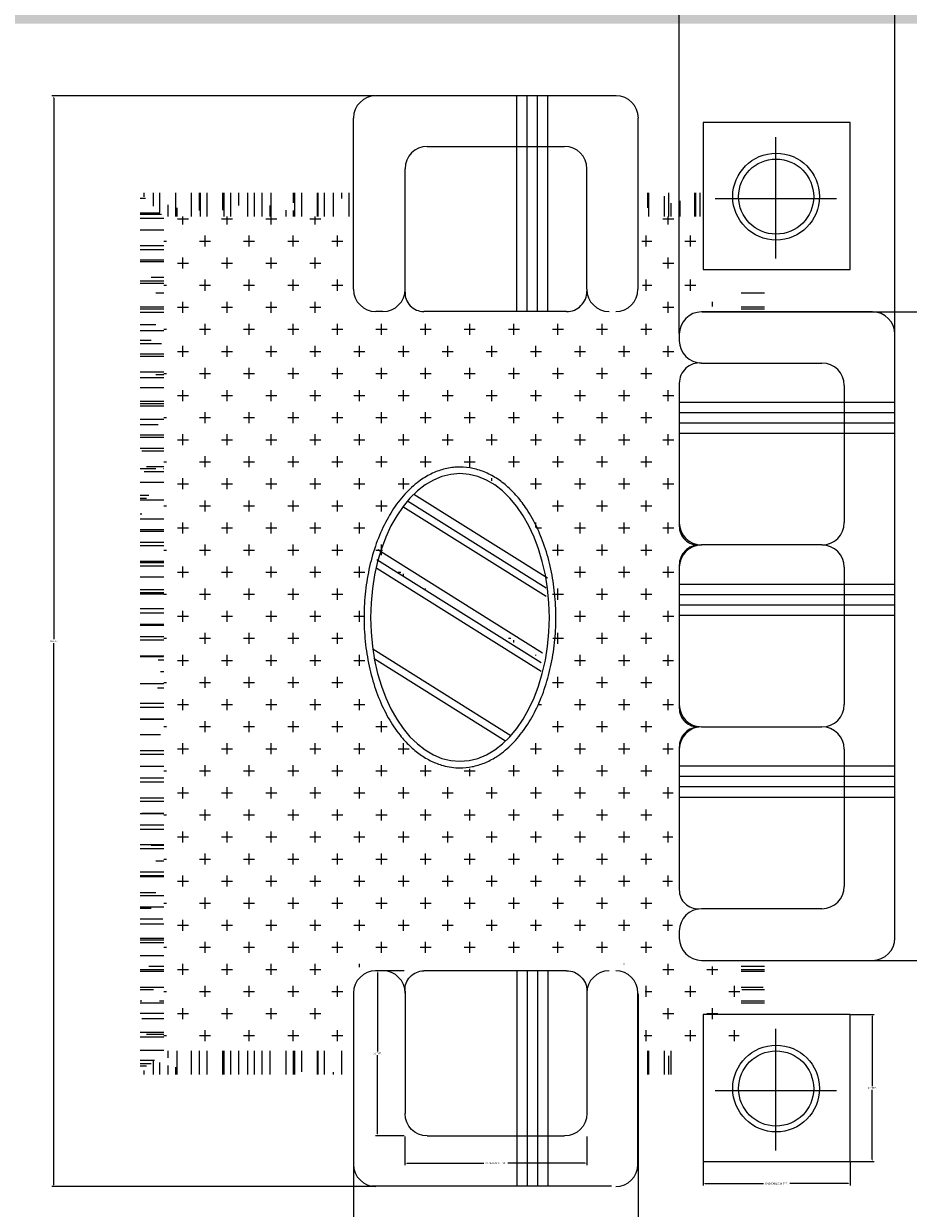
# Model space of a CAD drawing. Units: inches. Extents: x -30 to 437, y -29 to 647.
# Tile 12 of 15: x 308 to 392, y 321 to 435. Entities that reach past the tile are written whole.
import ezdxf

# ---------------------------------------------------------------- set-up
doc = ezdxf.new("R2010")
doc.units = ezdxf.units.IN
doc.header["$MEASUREMENT"] = 0
for name, color, linetype, lineweight in [('A-ANNO-DIMS', 2, 'Continuous', 18), ('A-FURN-PATT', 252, 'Continuous', 13), ('furniture', 220, 'Continuous', 18)]:
    doc.layers.add(name, color=color, linetype=linetype, lineweight=lineweight)
doc.layers.add('A-WALL-PATT', color=251, linetype='Continuous', lineweight=13, true_color=0x636466)
doc.styles.get("Standard").update_dxf_attribs({"font": 'arial.ttf'})
doc.dimstyles.get("Standard").update_dxf_attribs({"dimtxt": 0.18, "dimasz": 0.18, "dimexe": 0.18, "dimexo": 0.0625, "dimgap": 0.09, "dimtad": 0, "dimtih": 1, "dimtoh": 1, "dimdec": 4, "dimzin": 0, "dimdsep": 46, "dimtxsty": 'Standard', "dimcen": 0.09, "dimadec": 0, "dimazin": 0, "dimtfac": 1, "dimtdec": 4, "dimtofl": 0, "dimtmove": 0, "dimatfit": 3, "dimfxl": 1, "dimtolj": 1, "dimtzin": 0, "dimarcsym": 0})

# ---------------------------------------------------------------- blocks, each defined once
blk = doc.blocks.new('LOUNGE-CHAIR-CUSHION')
for p, q in [((2.14, 15.83), (15.3, 15.83)), ((0, 1.94), (0.01, 13.69)), ((17.44, 2.14), (17.44, 13.69)), ((15.5, 0), (1.8, 0))]:
    blk.add_line(p, q)
for centre, radius, start, end in [((2.14, 13.69), 2.14, 90, 180), ((15.3, 13.69), 2.14, 0, 90), ((1.8, 1.8), 1.8, 177.014, 270), ((15.52, 1.92), 1.92, 269.3411, 0.6299)]:
    blk.add_arc(centre, radius, start, end)
blk = doc.blocks.new('LOUNGE-END-TABLE')
for p, q in [((14.11, 14.11), (0, 14.11)), ((0, 14.11), (0, 0)), ((14.11, 0), (14.11, 14.11)), ((6.95, 12.71), (6.95, 1.07)), ((1.14, 6.81), (12.78, 6.81)), ((0, 0), (14.11, 0))]:
    blk.add_line(p, q)
for radius in [4.16, 3.6]:
    blk.add_circle((7, 7), radius)
blk = doc.blocks.new('*D15')
at = {"layer": 'A-ANNO-DIMS', "color": 0, "lineweight": -2, "transparency": 16777216}
for p, q in [((344.07, 327.86), (344.07, 325.12)), ((361.54, 327.86), (361.54, 325.12)), ((344.25, 325.3), (351.66, 325.3)), ((361.36, 325.3), (353.94, 325.3))]:
    blk.add_line(p, q, dxfattribs=at)
at = {"layer": 'A-ANNO-DIMS', "color": 0, "transparency": 16777216}
for points in [[(344.25, 325.33), (344.25, 325.27), (344.07, 325.3)], [(361.36, 325.33), (361.36, 325.27), (361.54, 325.3)]]:
    blk.add_solid(points, dxfattribs=at)
at = {"layer": 'Defpoints', "color": 0, "transparency": 16777216}
for p in [(344.07, 327.92), (361.54, 327.92), (361.54, 325.3)]:
    blk.add_point(p, dxfattribs=at)
at = {"layer": 'A-ANNO-DIMS', "color": 0, "transparency": 16777216, "insert": (352.8, 325.3), "char_height": 0.18, "attachment_point": 5}
blk.add_mtext('\\A1;CUSHION 17 TYP.', dxfattribs=at)
blk = doc.blocks.new('*D16')
at = {"layer": 'A-ANNO-DIMS', "color": 0, "lineweight": -2, "transparency": 16777216}
for p, q in [((344.01, 343.75), (341.27, 343.75)), ((341.45, 343.57), (341.45, 336.02)), ((341.45, 328.1), (341.45, 335.65)), ((344.01, 327.92), (341.27, 327.92))]:
    blk.add_line(p, q, dxfattribs=at)
at = {"layer": 'A-ANNO-DIMS', "color": 0, "transparency": 16777216}
for points in [[(341.42, 343.57), (341.48, 343.57), (341.45, 343.75)], [(341.42, 328.1), (341.48, 328.1), (341.45, 327.92)]]:
    blk.add_solid(points, dxfattribs=at)
at = {"layer": 'Defpoints', "color": 0, "transparency": 16777216}
for p in [(344.07, 343.75), (341.45, 327.92), (344.07, 327.92)]:
    blk.add_point(p, dxfattribs=at)
at = {"layer": 'A-ANNO-DIMS', "color": 0, "transparency": 16777216, "insert": (341.45, 335.83), "char_height": 0.18, "attachment_point": 5}
blk.add_mtext('\\A1;16 TYP.', dxfattribs=at)
blk = doc.blocks.new('*D17')
at = {"layer": 'A-ANNO-DIMS', "color": 0, "lineweight": -2, "transparency": 16777216}
for p, q in [((372.69, 325.4), (372.69, 323.16)), ((386.79, 325.4), (386.79, 323.16)), ((372.87, 323.34), (378.48, 323.34)), ((386.61, 323.34), (381, 323.34))]:
    blk.add_line(p, q, dxfattribs=at)
at = {"layer": 'A-ANNO-DIMS', "color": 0, "transparency": 16777216}
for points in [[(372.87, 323.37), (372.87, 323.31), (372.69, 323.34)], [(386.61, 323.37), (386.61, 323.31), (386.79, 323.34)]]:
    blk.add_solid(points, dxfattribs=at)
at = {"layer": 'Defpoints', "color": 0, "transparency": 16777216}
for p in [(372.69, 325.46), (386.79, 325.46), (386.79, 323.34)]:
    blk.add_point(p, dxfattribs=at)
at = {"layer": 'A-ANNO-DIMS', "color": 0, "transparency": 16777216, "insert": (379.74, 323.34), "char_height": 0.18, "attachment_point": 5}
blk.add_mtext('\\A1;END TABLE 14 TYP.', dxfattribs=at)
blk = doc.blocks.new('*D18')
at = {"layer": 'A-ANNO-DIMS', "color": 0, "lineweight": -2, "transparency": 16777216}
for p, q in [((386.86, 339.57), (389.09, 339.57)), ((388.91, 339.39), (388.91, 332.69)), ((388.91, 325.64), (388.91, 332.33)), ((386.86, 325.46), (389.09, 325.46))]:
    blk.add_line(p, q, dxfattribs=at)
at = {"layer": 'A-ANNO-DIMS', "color": 0, "transparency": 16777216}
for points in [[(388.88, 339.39), (388.94, 339.39), (388.91, 339.57)], [(388.88, 325.64), (388.94, 325.64), (388.91, 325.46)]]:
    blk.add_solid(points, dxfattribs=at)
at = {"layer": 'Defpoints', "color": 0, "transparency": 16777216}
for p in [(386.79, 339.57), (388.91, 339.57), (386.79, 325.46)]:
    blk.add_point(p, dxfattribs=at)
at = {"layer": 'A-ANNO-DIMS', "color": 0, "transparency": 16777216, "insert": (388.91, 332.51), "char_height": 0.18, "attachment_point": 5}
blk.add_mtext('\\A1;14 TYP.', dxfattribs=at)
blk = doc.blocks.new('*D47')
at = {"layer": 'A-ANNO-DIMS', "color": 0, "lineweight": -2, "transparency": 16777216}
for p, q in [((370.39, 404.84), (370.39, 435.86)), ((370.57, 435.68), (380.34, 435.68)), ((390.89, 435.68), (381.13, 435.68)), ((391.07, 404.84), (391.07, 435.86))]:
    blk.add_line(p, q, dxfattribs=at)
at = {"layer": 'A-ANNO-DIMS', "color": 0, "transparency": 16777216}
for points in [[(370.57, 435.71), (370.57, 435.65), (370.39, 435.68)], [(390.89, 435.71), (390.89, 435.65), (391.07, 435.68)]]:
    blk.add_solid(points, dxfattribs=at)
at = {"layer": 'Defpoints', "color": 0, "transparency": 16777216}
for p in [(391.07, 435.68), (370.39, 404.78), (391.07, 404.78)]:
    blk.add_point(p, dxfattribs=at)
at = {"layer": 'A-ANNO-DIMS', "color": 0, "transparency": 16777216, "insert": (380.73, 435.68), "char_height": 0.18, "attachment_point": 5}
blk.add_mtext('\\A1;20.68', dxfattribs=at)
blk = doc.blocks.new('*D48')
at = {"layer": 'A-ANNO-DIMS', "color": 0, "lineweight": -2, "transparency": 16777216}
for p, q in [((372.59, 406.91), (403.61, 406.91)), ((403.43, 406.73), (403.43, 376.01)), ((403.43, 344.92), (403.43, 375.65)), ((372.59, 344.74), (403.61, 344.74))]:
    blk.add_line(p, q, dxfattribs=at)
at = {"layer": 'A-ANNO-DIMS', "color": 0, "transparency": 16777216}
for points in [[(403.4, 406.73), (403.46, 406.73), (403.43, 406.91)], [(403.4, 344.92), (403.46, 344.92), (403.43, 344.74)]]:
    blk.add_solid(points, dxfattribs=at)
at = {"layer": 'Defpoints', "color": 0, "transparency": 16777216}
for p in [(372.53, 406.91), (372.53, 344.74), (403.43, 344.74)]:
    blk.add_point(p, dxfattribs=at)
at = {"layer": 'A-ANNO-DIMS', "color": 0, "transparency": 16777216, "insert": (403.43, 375.83), "char_height": 0.18, "attachment_point": 5}
blk.add_mtext('\\A1;62.17', dxfattribs=at)
blk = doc.blocks.new('*D49')
at = {"layer": 'A-ANNO-DIMS', "color": 0, "lineweight": -2, "transparency": 16777216}
for p, q in [((341.22, 427.63), (310.21, 427.63)), ((310.39, 427.45), (310.39, 375.53)), ((310.39, 323.24), (310.39, 375.17)), ((341.22, 323.06), (310.21, 323.06))]:
    blk.add_line(p, q, dxfattribs=at)
at = {"layer": 'A-ANNO-DIMS', "color": 0, "transparency": 16777216}
for points in [[(310.36, 427.45), (310.42, 427.45), (310.39, 427.63)], [(310.36, 323.24), (310.42, 323.24), (310.39, 323.06)]]:
    blk.add_solid(points, dxfattribs=at)
at = {"layer": 'Defpoints', "color": 0, "transparency": 16777216}
for p in [(310.39, 427.63), (341.29, 427.63), (341.29, 323.06)]:
    blk.add_point(p, dxfattribs=at)
at = {"layer": 'A-ANNO-DIMS', "color": 0, "transparency": 16777216, "insert": (310.39, 375.35), "char_height": 0.18, "attachment_point": 5}
blk.add_mtext('\\A1;104.57', dxfattribs=at)
blk = doc.blocks.new('*D50')
at = {"layer": 'A-ANNO-DIMS', "color": 0, "lineweight": -2, "transparency": 16777216}
for p, q in [((339.15, 341.54), (339.15, 310.53)), ((366.44, 341.54), (366.44, 310.53)), ((339.33, 310.71), (352.33, 310.71)), ((366.26, 310.71), (353.26, 310.71))]:
    blk.add_line(p, q, dxfattribs=at)
at = {"layer": 'A-ANNO-DIMS', "color": 0, "transparency": 16777216}
for points in [[(339.33, 310.74), (339.33, 310.68), (339.15, 310.71)], [(366.26, 310.74), (366.26, 310.68), (366.44, 310.71)]]:
    blk.add_solid(points, dxfattribs=at)
at = {"layer": 'Defpoints', "color": 0, "transparency": 16777216}
for p in [(339.15, 341.61), (366.44, 341.61), (339.15, 310.71)]:
    blk.add_point(p, dxfattribs=at)
at = {"layer": 'A-ANNO-DIMS', "color": 0, "transparency": 16777216, "insert": (352.79, 310.71), "char_height": 0.18, "attachment_point": 5}
blk.add_mtext('\\A1;27.286', dxfattribs=at)

msp = doc.modelspace()

# ---------------------------------------------------------------- hatches: boundary and pattern name
at = {"layer": 'A-FURN-PATT'}
h = msp.add_hatch(dxfattribs=at)
h.set_pattern_fill('AR-RROOF', color=256, scale=2.507942, angle=450, style=0)
h.set_pattern_definition([(360, (128.108, 59.7954), (4.965726, -2.257148), [33.85722, -4.5143, 11.28574, -2.25715]), (360, (131.11, 58.6668), (-2.257148, -3.002007), [6.771445, -0.74486, 13.54289, -1.69286]), (360, (129.2365, 57.8768), (11.7371705, -1.5122893), [18.057185, -3.16001, 9.028593, -2.25715])])
h.paths.add_polyline_path([(378.586, 408.8968), (378.586, 406.9147), (376.3288, 406.9147), (376.3288, 408.8968)])
h.paths.add_polyline_path([(320.9461, 416.0663), (320.9461, 336.0683), (318.6889, 333.8111), (318.6889, 418.3234)])
h.paths.add_polyline_path([(378.586, 344.7425), (378.586, 339.5062), (376.3288, 339.8024), (376.3288, 344.7425)])
h = msp.add_hatch(dxfattribs=at)
h.set_pattern_fill('AR-RROOF', color=256, scale=2.507942, angle=360, style=0)
h.set_pattern_definition([(90, (128.108, 59.7954), (2.257148, 4.965726), [33.85722, -4.5143, 11.28574, -2.25715]), (90, (129.2365, 62.7974), (3.002007, -2.257148), [6.771445, -0.74486, 13.54289, -1.69286]), (90, (130.0265, 60.924), (1.5122893, 11.7371705), [18.057185, -3.16001, 9.028593, -2.25715])])
h.paths.add_polyline_path([(372.6871, 418.3234), (372.6871, 416.0663), (366.4355, 416.0663), (366.4355, 418.3234)])
h.paths.add_polyline_path([(339.1493, 418.3234), (339.1493, 416.0663), (320.9461, 416.0663), (318.6889, 418.3234)])
h.paths.add_polyline_path([(339.1493, 336.0683), (339.1493, 333.8111), (318.6889, 333.8111), (320.9461, 336.0683)])
h.paths.add_polyline_path([(369.9519, 336.0683), (369.6551, 333.8111), (366.4355, 333.8111), (366.4355, 336.0683)])
h = msp.add_hatch(dxfattribs=at)
h.set_pattern_fill('CROSS', color=256, scale=9.404784, angle=360, style=0)
h.set_pattern_definition([(90, (128.108, 59.7954), (2.116076, 2.116076), [1.058038, -3.174115]), (360, (127.579, 60.3244), (2.116076, -2.116076), [1.058038, -3.174115])])
h.paths.add_polyline_path([(338.4543, 416.0663), (338.6819, 408.154), (338.8175, 406.526), (365.2559, 406.3904), (366.8829, 407.34), (366.7891, 416.0663), (372.6871, 416.0663), (372.6871, 408.8968), (376.3288, 408.8968), (376.3288, 407.5066), (370.0013, 407.34), (369.7301, 345.6144), (370.6792, 344.1221), (376.3288, 344.2006), (376.3288, 338.8335), (375.929, 336.0683), (367.005, 336.0683), (367.1541, 342.6298), (365.2559, 344.3934), (342.4782, 344.8004), (338.8175, 343.8508), (338.5666, 336.0683), (320.9461, 336.0683), (320.9461, 416.0663)])
h.paths.add_polyline_path([(340.9868, 379.5296), (341.1224, 369.4907), (345.7322, 363.9286), (347.7659, 363.1146), (350.3419, 363.1146), (352.2401, 363.5216), (354.8161, 364.7425), (355.9008, 367.3201), (357.3922, 370.3046), (358.0701, 373.5605), (358.4768, 377.4946), (356.9854, 385.77), (353.5959, 390.5181), (348.1726, 391.4677), (345.0542, 389.9754), (342.3426, 386.0413)], flags=16)
edge = h.paths.add_edge_path(flags=0)
edge.add_line((342.1946, 382.8659), (356.9997, 373.9636))
edge.add_ellipse((334.1097, 377.4396), major_axis=(16.3712, -16.3712), ratio=1, start_angle=35.87674, end_angle=36.365125, ccw=False)
edge.add_line((356.9692, 373.7686), (342.1504, 382.6792))
edge.add_ellipse((364.7022, 377.4396), major_axis=(-16.3712, -16.3712), ratio=1, start_angle=301.445378, end_angle=301.920237, ccw=False)
edge.add_line((342.1946, 382.8659), (342.1946, 382.8659))
edge.add_ellipse((357.1468, 379.2596), major_axis=(-10.876, -10.876), ratio=0.9999999, start_angle=301.439889, end_angle=301.456246)
edge.add_line((342.1936, 382.8616), (342.1936, 382.8616))
edge.add_line((342.1936, 382.8616), (342.1936, 382.8616))
edge.add_line((342.1936, 382.8616), (342.1936, 382.8616))
edge.add_line((342.1936, 382.8616), (342.1936, 382.8616))
edge.add_line((342.1936, 382.8616), (342.1936, 382.8616))
edge.add_ellipse((357.1468, 379.2596), major_axis=(10.876, -10.876), ratio=0.99999997, start_angle=211.439889, end_angle=211.456241, ccw=False)
at = {"layer": 'A-WALL-PATT'}
h = msp.add_hatch(color=256, dxfattribs=at)
h.dxf.hatch_style = 1
h.paths.add_polyline_path([(393.6054, 183.2352), (369.6054, 183.2352), (369.6054, 213.2352), (393.6054, 213.2352), (393.6054, 207.2352), (394.6054, 207.2352), (394.6054, 211.2352), (395.6054, 211.2352), (395.6054, 185.2352), (394.6054, 185.2352), (394.6054, 189.2352), (393.6054, 189.2352)], flags=0)
h.paths.add_polyline_path([(384.6054, 189.2352, -1), (390.6054, 189.2352, -1)], flags=0)
h.paths.add_polyline_path([(385.6054, 189.2352, -1), (389.6054, 189.2352, -1)], flags=0)
h.paths.add_polyline_path([(374.6054, 189.2352, -1), (382.6054, 189.2352, -1)], flags=0)
h.paths.add_polyline_path([(386.6054, 189.2352, -1), (388.6054, 189.2352, -1)], flags=0)
h.paths.add_polyline_path([(375.6054, 189.2352, -1), (381.6054, 189.2352, -1)], flags=0)
h.paths.add_polyline_path([(376.6054, 189.2352, -1), (380.6054, 189.2352, -1)], flags=0)
h.paths.add_polyline_path([(377.6054, 189.2352, -1), (379.6054, 189.2352, -1)], flags=0)
h.paths.add_polyline_path([(390.6054, 195.2352), (374.6054, 195.2352), (374.6054, 201.2352), (390.6054, 201.2352)], flags=0)
h.paths.add_polyline_path([(389.6054, 196.2352), (375.6054, 196.2352), (375.6054, 200.2352), (389.6054, 200.2352)], flags=0)
h.paths.add_polyline_path([(383.6054, 207.2352, -1), (391.6054, 207.2352, -1)], flags=0)
h.paths.add_polyline_path([(384.6054, 207.2352, -1), (390.6054, 207.2352, -1)], flags=0)
h.paths.add_polyline_path([(385.6054, 207.2352, -1), (389.6054, 207.2352, -1)], flags=0)
h.paths.add_polyline_path([(386.6054, 207.2352, -1), (388.6054, 207.2352, -1)], flags=0)
h.paths.add_polyline_path([(375.6054, 207.2352, -1), (381.6054, 207.2352, -1)], flags=0)
h.paths.add_polyline_path([(376.6054, 207.2352, -1), (380.6054, 207.2352, -1)], flags=0)
h.paths.add_polyline_path([(377.6054, 207.2352, -1), (379.6054, 207.2352, -1)], flags=0)
h.paths.add_polyline_path([(305.5437, 160.3663, -0.41421356), (304.0437, 158.8663), (271.0437, 158.8663, -0.41421356), (269.5437, 160.3663), (269.5437, 178.3663, -0.41421356), (271.0437, 179.8663), (304.0437, 179.8663, -0.41421356), (305.5437, 178.3663)], flags=0)
h.paths.add_polyline_path([(304.0437, 165.3663, -0.41421356), (303.0437, 164.3663), (289.2937, 164.3663, -0.41421356), (288.2937, 165.3663), (288.2937, 177.3663, -0.41421356), (289.2937, 178.3663), (303.0437, 178.3663, -0.41421356), (304.0437, 177.3663)], flags=0)
h.paths.add_polyline_path([(296.5437, 171.3663, -1), (295.5437, 171.3663, -1)], flags=0)
h.paths.add_polyline_path([(286.7937, 165.3663, -0.41421356), (285.7937, 164.3663), (272.0437, 164.3663, -0.41421356), (271.0437, 165.3663), (271.0437, 177.3663, -0.41421356), (272.0437, 178.3663), (285.7937, 178.3663, -0.41421356), (286.7937, 177.3663)], flags=0)
h.paths.add_polyline_path([(279.5437, 171.3663, -1), (278.5437, 171.3663, -1)], flags=0)
h.paths.add_polyline_path([(360.6737, 290.5474), (360.6737, 300.5474), (396.6737, 300.5474), (396.6737, 290.5474)], flags=0)
h.paths.add_polyline_path([(259.6737, 124.5474), (259.6737, 114.5474), (171.6737, 114.5474), (171.6737, 124.5474)], flags=0)
h.paths.add_polyline_path([(288.0737, 215.3705), (286.7097, 214.583), (268.7097, 245.7599), (270.0737, 246.5474)], flags=0)
h.paths.add_polyline_path([(259.6737, 168.5474), (256.6737, 168.5474), (256.6737, 173.5474), (256.6737, 179.0224), (255.8753, 177.6395), (224.2956, 195.872, 0.12053744), (220.1737, 179.0224, 0.12053744), (216.0518, 195.872), (184.4721, 177.6395), (183.6737, 179.0224), (215.2836, 197.2724), (216.0821, 195.8895), (216.0518, 195.872, -0.12053744), (220.1737, 179.0224, -0.12053744), (224.2956, 195.872), (224.2653, 195.8895), (225.0638, 197.2724), (256.6737, 179.0224), (256.6737, 173.5474), (259.6737, 173.5474)], flags=0)
h.paths.add_polyline_path([(386.7943, 325.4601), (372.6871, 325.4601), (372.6871, 339.5673), (386.7943, 339.5673)], flags=0)
h.paths.add_polyline_path([(359.5875, 343.7429), (357.7905, 343.7429), (357.7905, 327.9179), (359.3933, 327.9179, 0.41420885), (361.5302, 330.0549), (361.5302, 341.8434, 0.41436161)], flags=0)
h.paths.add_polyline_path([(341.7887, 323.1235, -0.11921667), (340.7839, 323.1235)], flags=0)
h.paths.add_polyline_path([(379.6332, 328.8632), (379.6332, 332.2699), (376.0992, 332.2699, 0.39427733)], flags=0)
h.paths.add_polyline_path([(375.5299, 332.459, -1), (383.8511, 332.459, -1)], flags=0)
h.paths.add_polyline_path([(388.9363, 344.7425), (372.5309, 344.7425, -0.41421356), (370.394, 346.8794), (370.394, 347.5594, -0.39085173), (372.3472, 349.7005, -0.43951011), (370.394, 351.4933), (370.394, 365.1894, -0.40305452), (372.2191, 367.1298, -0.41839453), (370.394, 368.9291), (370.394, 382.6251, -0.40885826), (372.2519, 384.5722, -0.42377324), (370.394, 386.3707), (370.394, 400.0667, -0.38660687), (372.1327, 402.0094), (372.531, 402.0094, -0.41421834), (370.394, 404.1464), (370.394, 404.7778, -0.41420891), (372.5309, 406.9147), (388.9363, 406.9147, -0.41421821), (391.0733, 404.7778), (391.0733, 346.8794, -0.41421356)], flags=0)
edge = h.paths.add_edge_path(flags=0)
edge.add_spline(control_points=[(349.3585, 363.204), (349.0859, 363.204), (348.8133, 363.2227), (348.2712, 363.2973), (348.0016, 363.3531), (347.3533, 363.5328), (346.9776, 363.6755), (346.2445, 364.0308), (345.887, 364.2432), (345.1953, 364.7329), (344.8611, 365.0101), (344.2197, 365.6237), (343.9125, 365.9603), (343.211, 366.8336), (342.8313, 367.3965), (342.1401, 368.6117), (341.8286, 369.2641), (341.2807, 370.64), (341.0443, 371.3636), (340.6522, 372.8619), (340.4964, 373.6367), (340.2695, 375.2158), (340.1983, 376.0203), (340.142, 377.6365), (340.157, 378.4483), (340.2729, 380.0567), (340.3738, 380.8533), (340.6589, 382.4093), (340.8432, 383.1686), (341.2906, 384.629), (341.5538, 385.3301), (342.1531, 386.6544), (342.4891, 387.2776), (343.2266, 388.4288), (343.6281, 388.9567), (344.4879, 389.9012), (344.9463, 390.3178), (345.7981, 390.9428), (346.182, 391.1771), (346.9712, 391.5648), (347.3766, 391.7182), (348.2004, 391.9387), (348.6189, 392.0058), (349.4588, 392.0508), (349.8801, 392.0288), (350.7146, 391.8966), (351.1278, 391.7865), (351.9366, 391.4822), (352.3323, 391.2882), (353.0989, 390.8223), (353.4699, 390.5504), (354.1819, 389.9355), (354.5229, 389.5924), (355.1706, 388.8418), (355.4772, 388.4343), (356.1315, 387.4422), (356.4671, 386.8397), (357.0692, 385.5581), (357.3356, 384.879), (357.7933, 383.4624), (357.9846, 382.725), (358.2875, 381.2112), (358.3992, 380.4349), (358.5404, 378.8643), (358.5699, 378.0699), (358.546, 376.4841), (358.4926, 375.6928), (358.3042, 374.1343), (358.1692, 373.3672), (357.8207, 371.8774), (357.6072, 371.1549), (357.1067, 369.7735), (356.8196, 369.1148), (356.1782, 367.8787), (355.8238, 367.3013), (355.0551, 366.244), (354.6408, 365.7641), (353.7607, 364.9161), (353.2948, 364.5481), (352.445, 364.0149), (352.0701, 363.822), (351.3034, 363.5117), (350.9116, 363.3943), (350.1325, 363.2418), (349.7455, 363.204), (349.3585, 363.204)], knot_values=[3.14159265, 3.14159265, 3.14159265, 3.14159265, 3.22691715, 3.22691715, 3.31224165, 3.31224165, 3.43426671, 3.43426671, 3.55629177, 3.55629177, 3.67831683, 3.67831683, 3.8003419, 3.8003419, 3.97157384, 3.97157384, 4.14280577, 4.14280577, 4.31403771, 4.31403771, 4.48526965, 4.48526965, 4.65650159, 4.65650159, 4.82773353, 4.82773353, 4.99896547, 4.99896547, 5.1701974, 5.1701974, 5.34142934, 5.34142934, 5.51266128, 5.51266128, 5.68389322, 5.68389322, 5.85512516, 5.85512516, 5.98669107, 5.98669107, 6.11825699, 6.11825699, 6.24982291, 6.24982291, 6.38138882, 6.38138882, 6.51295474, 6.51295474, 6.64452065, 6.64452065, 6.77608657, 6.77608657, 6.90765249, 6.90765249, 7.0392184, 7.0392184, 7.20701563, 7.20701563, 7.37481286, 7.37481286, 7.54261009, 7.54261009, 7.71040732, 7.71040732, 7.87820455, 7.87820455, 8.04600178, 8.04600178, 8.21379901, 8.21379901, 8.38159624, 8.38159624, 8.54939347, 8.54939347, 8.7171907, 8.7171907, 8.88498794, 8.88498794, 9.05278517, 9.05278517, 9.17820699, 9.17820699, 9.30362881, 9.30362881, 9.42477796, 9.42477796, 9.42477796, 9.42477796], degree=3, periodic=0)
edge.add_line((341.1696, 384.3006), (341.2012, 384.2808))
edge = h.paths.add_edge_path(flags=0)
edge.add_line((344.3353, 388.7801), (344.317, 388.7915))
edge.add_ellipse((349.3585, 377.6204), major_axis=(0, -13.7895), ratio=0.62186025, start_angle=-244.867444, end_angle=-124.769923)
h.paths.add_polyline_path([(163.6737, 163.1474), (132.4968, 145.1474), (131.7093, 146.5114), (162.8862, 164.5114)], flags=0)
h.paths.add_polyline_path([(366.4355, 409.0896, -0.41423669), (364.2985, 406.9525, -0.4913499), (361.5302, 408.8973), (361.5302, 420.6405, 0.41421356), (359.3932, 422.7775), (357.7905, 422.7775), (357.7905, 406.9525), (359.6317, 406.9525, 0.42741026), (361.5332, 408.9757, 0.39869469), (363.6672, 406.9525, 0.51958103), (366.4355, 409.0895)], flags=0)
h.paths.add_polyline_path([(386.7943, 410.9671), (372.6871, 410.9671), (372.6871, 425.0742), (386.7943, 425.0742)], flags=0)
h.paths.add_polyline_path([(379.6332, 414.3701), (379.6332, 417.7768), (376.0992, 417.7768, 0.39427733)], flags=0)
h.paths.add_polyline_path([(375.5299, 417.966, -1), (383.8511, 417.966, -1)], flags=0)
h.paths.add_polyline_path([(150.0377, 351.583), (148.6737, 352.3705), (166.6737, 383.5474), (168.0377, 382.7599)], flags=0)
h.paths.add_polyline_path([(91.6737, 234.1974), (66.559, 219.6974), (65.9246, 220.7962), (91.0393, 235.2962)], flags=0)
h.paths.add_polyline_path([(255.4612, 443.5834), (254.6737, 444.9474), (285.8506, 462.9474), (286.6381, 461.5834)], flags=0)
h.paths.add_polyline_path([(176.2737, 394.5474), (158.2737, 425.7243), (159.6377, 426.5118), (177.6377, 395.3349)], flags=0)
h.paths.add_polyline_path([(243.6737, 439.5474), (243.0393, 438.4486), (217.9246, 452.9486), (218.559, 454.0474)], flags=0)
h.paths.add_polyline_path([(38.1264, 269.8429), (40.2408, 269.8429), (40.2408, 270.3508), (38.1264, 270.3508)], flags=0)
h.paths.add_polyline_path([(75.7157, 289.9439), (40.2408, 289.9439), (38.1264, 289.6524), (40.2408, 289.6524)], flags=0)
h.paths.add_polyline_path([(75.7157, 270.0846), (77.6447, 270.0846), (77.6697, 270.1626), (75.7175, 270.1626)], flags=0)
h.paths.add_polyline_path([(80.5373, 293.3002), (33.0467, 293.3002), (13.5054, 293.3002), (13.5054, 351.9244), (29.7898, 351.9244), (80.5373, 351.9244)], flags=0)
h.paths.add_polyline_path([(46.0261, 212.466, -0.50131678), (27.1651, 207.5106), (21.165, 209.5107), (21.165, 206.5107), (22.665, 206.5107), (22.665, 203.5107), (21.165, 203.5107), (21.165, 203.0107), (13.165, 203.0107), (13.165, 224.0107), (21.165, 224.0107), (21.165, 217.5107), (27.1649, 219.5106, -0.50132349), (46.0261, 214.5554, -0.13289091)], flags=0)
h.paths.add_polyline_path([(44.688, 211.8666, -0.48007965), (27.165, 209.5107), (27.165, 217.5107, -0.4800795), (44.688, 215.1547, -0.21500378)], flags=0)
h.paths.add_polyline_path([(19.415, 204.0107), (15.165, 204.0107, -0.41421356), (14.165, 204.7607), (14.165, 222.0107, -0.41421356), (14.915, 223.0107), (19.165, 223.0107, -0.41421356), (20.165, 222.2607), (20.165, 205.0107, -0.41421356)], flags=0)
h.paths.add_polyline_path([(32.7608, 269.0719), (31.8439, 269.0719), (31.8439, 268.6134), (13.5054, 268.6134), (13.5054, 291.5366), (31.8439, 291.5366), (32.7608, 291.0781), (32.7608, 280.9919, -1), (32.7608, 279.1581)], flags=0)
h.paths.add_polyline_path([(40.2408, 360.1436), (38.1264, 360.1436), (38.1264, 359.6357), (40.2408, 359.6357)], flags=0)
h.paths.add_polyline_path([(75.7157, 355.2807), (40.2408, 355.2807), (38.1264, 355.5722), (40.2408, 355.5722), (40.2408, 355.2807), (75.7157, 355.2807), (75.7157, 375.5982), (40.2408, 375.5982), (38.1264, 375.3817), (40.2408, 375.3817), (40.2408, 375.5982), (75.7157, 375.5982), (77.9733, 375.062), (75.7175, 375.062), (75.7175, 374.554)], flags=0)
h.paths.add_polyline_path([(42.8174, 299.814, 0.13867074), (34.1602, 294.603), (14.8081, 294.603), (14.8081, 350.6216), (29.8539, 350.6216, 0.09822056)], flags=0)
h.paths.add_polyline_path([(15.8636, 276.7781, -0.30640166), (20.3757, 283.4499), (20.3483, 290.6726), (31.4014, 290.7146), (31.4309, 282.9124), (26.8287, 282.895, -0.26006276), (30.241, 276.7781, -1)], flags=0)
h.paths.add_polyline_path([(26.1332, 276.7781), (23.0523, 273.6972), (19.9714, 276.7781), (23.0523, 279.8589), (23.0523, 283.9209), (21.3493, 283.9145), (20.7006, 283.5219), (20.6907, 286.1226), (23.2914, 286.1325), (25.8936, 285.7522), (27.1939, 285.7572), (28.4928, 286.1522), (31.0935, 286.1621), (31.0918, 286.6172), (25.6303, 286.5965), (25.616, 290.3675), (31.0775, 290.3882), (31.0918, 286.6172), (31.1034, 283.5614), (28.5027, 283.5515), (25.9005, 283.9317), (23.0523, 283.9209), (23.0523, 279.8589)], flags=0)
h.paths.add_polyline_path([(24.0793, 276.7781, -1), (22.0253, 276.7781, -1)], flags=0)
h.paths.add_polyline_path([(35.7687, 302.2895, -0.41421356), (35.2283, 301.2726), (22.2164, 297.2909, -0.41421356), (21.1995, 297.8313), (15.7317, 315.6996, -0.41421356), (16.2721, 316.7165), (18.8554, 317.507), (15.3721, 328.8904, -0.41421356), (15.9125, 329.9073), (28.9244, 333.889, -0.41421356), (29.9414, 333.3486), (35.4091, 315.4802, -0.41421356), (34.8687, 314.4633), (32.2854, 313.6728)], flags=0)
h.paths.add_polyline_path([(361.3728, 532.6207), (302.7487, 532.6207), (302.7487, 580.1113), (302.7487, 599.6527), (361.3728, 599.6527), (361.3728, 583.3682)], flags=0)
h.paths.add_polyline_path([(370.1, 575.0316), (370.1, 572.9172), (370.6079, 572.9172), (370.6079, 575.0316)], flags=0)
h.paths.add_polyline_path([(385.0466, 537.4423), (385.0466, 572.9172), (384.8302, 575.0316), (384.8302, 572.9172)], flags=0)
h.paths.add_polyline_path([(384.5104, 535.3262), (384.5104, 537.4406), (384.0025, 537.4406), (364.7291, 537.4423), (364.7291, 572.9172), (365.0206, 575.0316), (365.0206, 572.9172), (364.7291, 572.9172), (364.7291, 537.4423), (384.5884, 537.4423), (384.5884, 535.5133)], flags=0)
h.paths.add_polyline_path([(384.5884, 535.5133), (383.4945, 535.164), (383.4945, 537.4406), (382.9866, 535.3262), (382.9866, 537.4406), (383.4945, 535.3262), (383.4945, 537.4406), (384.5884, 537.4406)], flags=0)
h.paths.add_polyline_path([(23.874, 286.8174), (21.0132, 286.8065), (21.0004, 290.1875), (23.8612, 290.1983)], flags=0)
h.paths.add_polyline_path([(242.9824, 511.1667), (234.9824, 511.1667), (234.9824, 517.6667), (228.9825, 515.6667, -0.50132349), (210.1213, 520.622, -0.13289091), (210.1213, 522.7114, -0.50131678), (228.9823, 527.6667), (234.9824, 525.6667), (234.9824, 528.6667), (233.4824, 528.6667), (233.4824, 531.6667), (234.9824, 531.6667), (234.9824, 532.1667), (242.9824, 532.1667)], flags=0)
h.paths.add_polyline_path([(236.9824, 512.1667, -0.41421356), (235.9824, 512.9167), (235.9824, 530.1667, -0.41421356), (236.7324, 531.1667), (240.9824, 531.1667, -0.41421356), (241.9824, 530.4167), (241.9824, 513.1667, -0.41421356), (241.2324, 512.1667)], flags=0)
h.paths.add_polyline_path([(279.533, 537.4423), (279.533, 535.5133), (279.6111, 535.4884), (279.6111, 537.4406)], flags=0)
h.paths.add_polyline_path([(279.2913, 575.0316), (279.2913, 572.9172), (279.7992, 572.9172), (279.7992, 575.0316)], flags=0)
h.paths.add_polyline_path([(211.4594, 520.0227, -0.21500378), (211.4594, 523.3107, -0.48007965), (228.9824, 525.6667), (228.9824, 517.6667, -0.4800795)], flags=0)
h.paths.add_polyline_path([(32.7627, 354.1465), (31.8457, 354.1465), (31.8457, 353.688), (13.5054, 353.688), (13.5054, 376.6134), (31.8457, 376.6134), (32.7627, 376.1549), (32.7627, 366.0677, -1), (32.7627, 364.2337)], flags=0)
h.paths.add_polyline_path([(15.9446, 365.1507, -1), (30.3234, 365.1507, -1)], flags=0)
h.paths.add_polyline_path([(41.213, 428.467), (43.3274, 428.467), (43.3274, 428.9749), (41.213, 428.9749)], flags=0)
h.paths.add_polyline_path([(78.8022, 448.568), (43.3274, 448.568), (41.213, 448.2765), (43.3274, 448.2765)], flags=0)
h.paths.add_polyline_path([(78.8022, 428.7087), (80.7313, 428.7087), (80.7562, 428.7868), (78.804, 428.7868)], flags=0)
h.paths.add_polyline_path([(26.2152, 365.1507), (23.134, 362.0696), (20.0529, 365.1507), (23.134, 368.2319)], flags=0)
h.paths.add_polyline_path([(24.1611, 365.1507, -1), (22.107, 365.1507, -1)], flags=0)
h.paths.add_polyline_path([(309.2625, 570.3406, 0.13867074), (304.0514, 578.9978), (304.0514, 598.3499), (360.07, 598.3499), (360.07, 583.3041, 0.09822056)], flags=0)
h.paths.add_polyline_path([(246.6737, 552.5474), (129.6737, 552.5474), (129.6737, 606.5474), (246.6737, 606.5474)], flags=16)
h.paths.add_polyline_path([(373.6822, 580.3953), (363.595, 580.3953), (363.595, 581.3123), (363.1365, 581.3123), (363.1365, 599.6527), (386.0619, 599.6527), (386.0619, 581.3123), (385.6034, 580.3953), (375.5162, 580.3953, -1)], flags=0)
h.paths.add_polyline_path([(83.6239, 451.9244), (36.1333, 451.9244), (16.5919, 451.9244), (16.5919, 510.5485), (32.8764, 510.5485), (83.6239, 510.5485)], flags=0)
h.paths.add_polyline_path([(367.4098, 590.024, -1), (381.7886, 590.024, -1)], flags=0)
h.paths.add_polyline_path([(374.5992, 586.9428), (371.518, 590.024), (374.5992, 593.1052), (377.6803, 590.024)], flags=0)
h.paths.add_polyline_path([(373.5721, 590.024, -1), (375.6262, 590.024, -1)], flags=0)
h.paths.add_polyline_path([(324.9287, 577.7489, -0.41421356), (323.9118, 578.2893), (323.1212, 580.8726), (311.7379, 577.3893, -0.41421356), (310.721, 577.9297), (306.7393, 590.9416, -0.41421356), (307.2797, 591.9585), (325.1481, 597.4263, -0.41421356), (326.165, 596.8859), (326.9555, 594.3026), (338.3388, 597.7859, -0.41421356), (339.3557, 597.2455), (343.3374, 584.2336, -0.41421356), (342.797, 583.2167)], flags=0)
h.paths.add_polyline_path([(300.5265, 580.3972), (290.4404, 580.3972, -1), (288.6065, 580.3972), (278.5203, 580.3972), (278.5203, 581.3142), (278.0619, 581.3142), (278.0619, 599.6527), (300.985, 599.6527), (300.985, 581.3142)], flags=0)
h.paths.add_polyline_path([(300.163, 581.7567), (292.3609, 581.7271), (292.3434, 586.3294, -0.75567924), (279.0378, 590.1057, -0.82536731), (292.8983, 592.7823), (300.1211, 592.8097)], flags=0)
h.paths.add_polyline_path([(299.8367, 582.0805), (296.0656, 582.0662), (293.0098, 582.0546), (292.9999, 584.6553), (293.3802, 587.2575), (293.3694, 590.1057), (289.3074, 590.1057), (286.2265, 587.0248), (283.1456, 590.1057), (286.2265, 593.1866), (289.3074, 590.1057), (293.3694, 590.1057), (293.3629, 591.8088), (292.9703, 592.4575), (295.5711, 592.4673), (295.5809, 589.8666), (295.2007, 587.2644), (295.2056, 585.9641), (295.6006, 584.6652), (295.6105, 582.0645), (296.0656, 582.0662), (296.0449, 587.5277), (299.8159, 587.542)], flags=0)
h.paths.add_polyline_path([(285.1995, 590.1057, -1), (287.2535, 590.1057, -1)], flags=0)
h.paths.add_polyline_path([(299.6467, 589.2969), (296.2658, 589.284), (296.255, 592.1448), (299.6359, 592.1576)], flags=0)
h.paths.add_polyline_path([(35.8473, 427.696), (34.9304, 427.696), (34.9304, 427.2376), (16.5919, 427.2376), (16.5919, 450.1607), (34.9304, 450.1607), (35.8473, 449.7022), (35.8473, 439.6161, -1), (35.8473, 437.7822)], flags=0)
h.paths.add_polyline_path([(18.9502, 435.4022, -0.30640166), (23.4623, 442.074), (23.4349, 449.2968), (34.4879, 449.3387), (34.5175, 441.5366), (29.9152, 441.5191, -0.26006276), (33.3275, 435.4022, -1)], flags=0)
h.paths.add_polyline_path([(29.2197, 435.4022), (26.1389, 432.3213), (23.058, 435.4022), (26.1389, 438.4831), (26.1389, 442.5451), (24.4358, 442.5386), (23.7871, 442.1461), (23.7772, 444.7468), (26.378, 444.7566), (28.9801, 444.3764), (30.2805, 444.3813), (31.5794, 444.7764), (34.1801, 444.7862), (34.1784, 445.2413), (28.7169, 445.2206), (28.7026, 448.9917), (34.164, 449.0124), (34.1784, 445.2413), (34.1899, 442.1855), (31.5892, 442.1756), (28.987, 442.5559), (26.1389, 442.5451), (26.1389, 438.4831)], flags=0)
h.paths.add_polyline_path([(27.1658, 435.4022, -1), (25.1119, 435.4022, -1)], flags=0)
h.paths.add_polyline_path([(45.904, 458.4382, 0.13867074), (37.2467, 453.2271), (17.8947, 453.2271), (17.8947, 509.2457), (32.9405, 509.2457, 0.09822056)], flags=0)
h.paths.add_polyline_path([(26.9605, 445.4415), (24.0997, 445.4307), (24.0869, 448.8116), (26.9477, 448.8225)], flags=0)
h.paths.add_polyline_path([(38.3149, 459.8967), (25.3029, 455.915, -0.41421356), (24.286, 456.4554), (18.8183, 474.3238, -0.41421356), (19.3586, 475.3407), (21.942, 476.1312), (18.4587, 487.5145, -0.41421356), (18.999, 488.5314), (32.011, 492.5131, -0.41421356), (33.0279, 491.9727), (38.4957, 474.1044, -0.41421356), (37.9553, 473.0875), (35.3719, 472.297), (38.8553, 460.9136, -0.41421356)], flags=0)
h.paths.add_polyline_path([(43.3274, 518.7678), (41.213, 518.7678), (41.213, 518.2598), (43.3274, 518.2598)], flags=0)
h.paths.add_polyline_path([(78.8022, 513.9049), (43.3274, 513.9049), (41.213, 514.1964), (43.3274, 514.1964), (43.3274, 513.9049), (78.8022, 513.9049), (78.8022, 534.2223), (43.3274, 534.2223), (41.213, 534.0059), (43.3274, 534.0059), (43.3274, 534.2223), (78.8022, 534.2223), (81.0599, 533.6861), (78.804, 533.6861), (78.804, 533.1782)], flags=0)
h.paths.add_polyline_path([(121.6737, 556.8974), (121.0393, 555.7986), (95.9246, 570.2986), (96.559, 571.3974)], flags=0)
h.paths.add_polyline_path([(35.8493, 512.7707), (34.9322, 512.7707), (34.9322, 512.3122), (16.5919, 512.3122), (16.5919, 535.2376), (34.9322, 535.2376), (35.8493, 534.7791), (35.8493, 524.6919, -1), (35.8493, 522.8579)], flags=0)
h.paths.add_polyline_path([(19.0312, 523.7749, -1), (33.41, 523.7749, -1)], flags=0)
h.paths.add_polyline_path([(26.2206, 520.6937), (23.1394, 523.7749), (26.2206, 526.8561), (29.3018, 523.7749)], flags=0)
h.paths.add_polyline_path([(25.1935, 523.7749, -1), (27.2476, 523.7749, -1)], flags=0)
h.paths.add_polyline_path([(28.4381, 586.0173), (22.438, 588.0173), (22.438, 585.0173), (23.938, 585.0173), (23.938, 582.0173), (22.438, 582.0173), (22.438, 581.5173), (14.438, 581.5173), (14.438, 602.5173), (22.438, 602.5173), (22.438, 596.0173), (28.4379, 598.0173, -0.50132349), (47.2992, 593.062, -0.13289091), (47.2992, 590.9726, -0.50131678)], flags=0)
h.paths.add_polyline_path([(28.438, 588.0174), (28.438, 596.0173, -0.4800795), (45.961, 593.6614, -0.21500378), (45.961, 590.3733, -0.48007965)], flags=0)
h.paths.add_polyline_path([(20.688, 582.5173), (16.438, 582.5173, -0.41421356), (15.438, 583.2673), (15.438, 600.5173, -0.41421356), (16.188, 601.5173), (20.438, 601.5173, -0.41421356), (21.438, 600.7673), (21.438, 583.5173, -0.41421356)], flags=0)
h.paths.add_polyline_path([(171.6737, 2.0474), (171.6737, 104.5474), (259.6737, 104.5474), (259.6737, 148.5474), (396.6737, 148.5474), (396.6737, 2.0474), (405.6737, 2.0474), (405.6737, 615.5474), (1.6737, 615.5474), (1.6737, 2.0474)])
h.paths.add_polyline_path([(171.6737, 104.5474), (259.6737, 104.5474), (259.6737, 210.5474), (264.6737, 210.5474), (264.6737, 153.5474), (396.6737, 153.5474), (396.6737, 249.5474), (264.6737, 249.5474), (264.6737, 246.5474), (259.6737, 246.5474), (259.6737, 254.5474), (396.6737, 254.5474), (396.6737, 434.5474), (290.6737, 434.5474), (290.6737, 439.5474), (396.6737, 439.5474), (396.6737, 606.5474), (251.6737, 606.5474), (251.6737, 439.5474), (254.6737, 439.5474), (254.6737, 434.5474), (243.6737, 434.5474), (243.6737, 439.5474), (246.6737, 439.5474), (246.6737, 547.5474), (186.6737, 547.5474), (186.6737, 439.5474), (214.6737, 439.5474), (214.6737, 434.5474), (186.6737, 434.5474), (186.6737, 430.5474), (181.6737, 430.5474), (181.6737, 547.5474), (121.6737, 547.5474), (121.6737, 552.5474), (124.6737, 552.5474), (124.6737, 606.5474), (10.6737, 606.5474), (10.6737, 552.5474), (92.6737, 552.5474), (92.6737, 547.5474), (10.6737, 547.5474), (10.6737, 391.5474), (181.6737, 391.5474), (181.6737, 394.5474), (186.6737, 394.5474), (186.6737, 386.5474), (171.6737, 386.5474), (171.6737, 383.5474), (166.6737, 383.5474), (166.6737, 386.5474), (10.6737, 386.5474), (10.6737, 238.5474), (62.6737, 238.5474), (62.6737, 233.5474), (10.6737, 233.5474), (10.6737, 173.5474), (94.6737, 173.5474), (94.6737, 233.5474), (91.6737, 233.5474), (91.6737, 238.5474), (166.6737, 238.5474), (166.6737, 347.5474), (171.6737, 347.5474), (171.6737, 233.5474), (99.6737, 233.5474), (99.6737, 173.5474), (127.6737, 173.5474), (127.6737, 168.5474), (10.6737, 168.5474), (10.6737, 11.0474), (166.6737, 11.0474), (166.6737, 168.5474), (163.6737, 168.5474), (163.6737, 173.5474), (183.6737, 173.5474), (183.6737, 168.5474), (171.6737, 168.5474)])

# ---------------------------------------------------------------- linework, layer by layer
at = {"layer": 'furniture'}
for p, q in [((364.3471, 427.6318), (341.3261, 427.6318)), ((354.8043, 407.001), (354.8043, 427.6318)), ((355.7997, 407.001), (355.7997, 427.6318)), ((356.7951, 407.001), (356.7951, 427.6318)), ((357.7905, 407.001), (357.7905, 427.6318)), ((339.1493, 409.0895), (339.1493, 425.4948)), ((366.4355, 425.4948), (366.4355, 409.0895)), ((341.9662, 406.9525), (341.2863, 406.9525)), ((388.9363, 406.9147), (372.5309, 406.9147)), ((370.394, 404.7778), (370.394, 404.1464)), ((391.0733, 346.8794), (391.0733, 404.7778)), ((372.5309, 402.0094), (384.082, 402.0094)), ((370.394, 400.0667), (370.394, 386.3707)), ((386.219, 399.8725), (386.219, 386.7107)), ((370.4425, 398.2697), (391.0733, 398.2697)), ((370.4425, 397.2743), (391.0733, 397.2743)), ((370.4425, 396.2789), (391.0733, 396.2789)), ((370.4425, 395.2835), (391.0733, 395.2835)), ((357.6248, 380.4445), (344.3262, 388.7857)), ((357.7425, 381.3869), (344.9266, 389.4254)), ((357.6248, 379.6198), (343.8862, 388.2371)), ((357.2716, 374.2009), (341.4952, 384.0964)), ((384.082, 384.5737), (372.5309, 384.5737)), ((357.1539, 373.2585), (341.3774, 383.1539)), ((357.1539, 372.4339), (341.3774, 382.3293)), ((370.394, 382.6251), (370.394, 368.9291)), ((386.219, 382.4308), (386.219, 369.269)), ((370.4425, 380.8281), (391.0733, 380.8281)), ((370.4425, 379.8327), (391.0733, 379.8327)), ((370.4425, 378.8373), (391.0733, 378.8373)), ((370.4425, 377.8419), (391.0733, 377.8419)), ((354.2355, 366.2784), (340.9938, 374.5839)), ((353.7385, 365.7655), (341.1436, 373.6653)), ((372.5309, 367.1321), (384.082, 367.1321)), ((370.394, 365.1894), (370.394, 351.4933)), ((386.219, 364.9951), (386.219, 351.8333)), ((370.4425, 363.3924), (391.0733, 363.3924)), ((370.4425, 362.397), (391.0733, 362.397)), ((370.4425, 361.4016), (391.0733, 361.4016)), ((370.4425, 360.4062), (391.0733, 360.4062)), ((384.082, 349.6963), (372.5309, 349.6963)), ((370.394, 347.5594), (370.394, 346.7764)), ((372.5309, 344.7425), (388.9363, 344.7425)), ((341.9662, 343.7429), (341.2863, 343.7429)), ((354.8043, 343.6944), (354.8043, 323.0636)), ((355.7997, 343.6944), (355.7997, 323.0636)), ((356.7951, 343.6944), (356.7951, 323.0636)), ((357.7905, 343.6944), (357.7905, 323.0636)), ((339.1493, 341.606), (339.1493, 325.2006)), ((366.4355, 325.2006), (366.4355, 341.606)), ((340.8665, 323.1235), (363.8875, 323.1235))]:
    msp.add_line(p, q, dxfattribs=at)
for centre, radius, start, end in [((341.2863, 425.4948), 2.137, 90, 180), ((364.3384, 425.4948), 2.137, 0, 90), ((341.2863, 409.0895), 2.137, 180, 270), ((341.9662, 409.0895), 2.137, 270, 0), ((363.6672, 409.0895), 2.137, 180, 270), ((364.2985, 409.0895), 2.137, 270, 0), ((372.5309, 404.7778), 2.137, 90, 180), ((388.9363, 404.7778), 2.137, 0, 90), ((372.5309, 404.1464), 2.137, 180, 270), ((372.3318, 400.0818), 1.9379, 84.101853, 180.445527), ((384.082, 399.8725), 2.137, 0, 90), ((372.5309, 386.7048), 2.137, 180, 270), ((372.1934, 386.3707), 1.7994, 180, 272.985951), ((384.082, 386.7107), 2.137, 270, 0), ((372.3146, 382.6472), 1.9207, 89.370084, 180.65888), ((372.5309, 382.4367), 2.137, 90, 180), ((384.082, 382.4308), 2.137, 0, 90), ((372.5309, 369.269), 2.137, 180, 270), ((384.082, 369.269), 2.137, 270, 0), ((372.1934, 368.9291), 1.7994, 180, 272.985951), ((372.3146, 365.2115), 1.9207, 89.370084, 180.65888), ((372.5309, 364.9951), 2.137, 90, 180), ((384.082, 364.9951), 2.137, 0, 90), ((372.1934, 351.4933), 1.7994, 180, 272.985951), ((384.082, 351.8333), 2.137, 270, 0), ((372.5309, 347.5594), 2.137, 90, 180), ((372.5309, 346.8794), 2.137, 180, 270), ((388.9363, 346.8794), 2.137, 270, 0), ((341.2863, 341.606), 2.137, 90, 180), ((341.9662, 341.606), 2.137, 0, 90), ((363.6672, 341.606), 2.137, 90, 180), ((364.2985, 341.606), 2.137, 0, 90), ((341.2863, 325.2006), 2.137, 180, 270), ((364.2985, 325.2006), 2.137, 270, 0)]:
    msp.add_arc(centre, radius, start, end, dxfattribs=at)
at = {"layer": 'furniture', "extrusion": (0, 0, -1)}
msp.add_ellipse((349.3585, 377.6204), major_axis=(0, -13.7895), ratio=0.62186025, start_param=4.71238898, end_param=10.99557429, dxfattribs=at)
at = {"layer": 'furniture'}
msp.add_open_spline([(349.3585, 363.204), (349.0859, 363.204), (348.8133, 363.2227), (348.2712, 363.2973), (348.0016, 363.3531), (347.3533, 363.5328), (346.9776, 363.6755), (346.2445, 364.0308), (345.887, 364.2432), (345.1953, 364.7329), (344.8611, 365.0101), (344.2197, 365.6237), (343.9125, 365.9603), (343.211, 366.8336), (342.8313, 367.3965), (342.1401, 368.6117), (341.8286, 369.2641), (341.2807, 370.64), (341.0443, 371.3636), (340.6522, 372.8619), (340.4964, 373.6367), (340.2695, 375.2158), (340.1983, 376.0203), (340.142, 377.6365), (340.157, 378.4483), (340.2729, 380.0567), (340.3738, 380.8533), (340.6589, 382.4093), (340.8432, 383.1686), (341.2906, 384.629), (341.5538, 385.3301), (342.1531, 386.6544), (342.4891, 387.2776), (343.2266, 388.4288), (343.6281, 388.9567), (344.4879, 389.9012), (344.9463, 390.3178), (345.7981, 390.9428), (346.182, 391.1771), (346.9712, 391.5648), (347.3766, 391.7182), (348.2004, 391.9387), (348.6189, 392.0058), (349.4588, 392.0508), (349.8801, 392.0288), (350.7146, 391.8966), (351.1278, 391.7865), (351.9366, 391.4822), (352.3323, 391.2882), (353.0989, 390.8223), (353.4699, 390.5504), (354.1819, 389.9355), (354.5229, 389.5924), (355.1706, 388.8418), (355.4772, 388.4343), (356.1315, 387.4422), (356.4671, 386.8397), (357.0692, 385.5581), (357.3356, 384.879), (357.7933, 383.4624), (357.9846, 382.725), (358.2875, 381.2112), (358.3992, 380.4349), (358.5404, 378.8643), (358.5699, 378.0699), (358.546, 376.4841), (358.4926, 375.6928), (358.3042, 374.1343), (358.1692, 373.3672), (357.8207, 371.8774), (357.6072, 371.1549), (357.1067, 369.7735), (356.8196, 369.1148), (356.1782, 367.8787), (355.8238, 367.3013), (355.0551, 366.244), (354.6408, 365.7641), (353.7607, 364.9161), (353.2948, 364.5481), (352.445, 364.0149), (352.0701, 363.822), (351.3034, 363.5117), (350.9116, 363.3943), (350.1325, 363.2418), (349.7455, 363.204), (349.3585, 363.204)], degree=3, knots=[3.14159265, 3.14159265, 3.14159265, 3.14159265, 3.22691715, 3.22691715, 3.31224165, 3.31224165, 3.43426671, 3.43426671, 3.55629177, 3.55629177, 3.67831683, 3.67831683, 3.8003419, 3.8003419, 3.97157384, 3.97157384, 4.14280577, 4.14280577, 4.31403771, 4.31403771, 4.48526965, 4.48526965, 4.65650159, 4.65650159, 4.82773353, 4.82773353, 4.99896547, 4.99896547, 5.1701974, 5.1701974, 5.34142934, 5.34142934, 5.51266128, 5.51266128, 5.68389322, 5.68389322, 5.85512516, 5.85512516, 5.98669107, 5.98669107, 6.11825699, 6.11825699, 6.24982291, 6.24982291, 6.38138882, 6.38138882, 6.51295474, 6.51295474, 6.64452065, 6.64452065, 6.77608657, 6.77608657, 6.90765249, 6.90765249, 7.0392184, 7.0392184, 7.20701563, 7.20701563, 7.37481286, 7.37481286, 7.54261009, 7.54261009, 7.71040732, 7.71040732, 7.87820455, 7.87820455, 8.04600178, 8.04600178, 8.21379901, 8.21379901, 8.38159624, 8.38159624, 8.54939347, 8.54939347, 8.7171907, 8.7171907, 8.88498794, 8.88498794, 9.05278517, 9.05278517, 9.17820699, 9.17820699, 9.30362881, 9.30362881, 9.42477796, 9.42477796, 9.42477796, 9.42477796], dxfattribs=at)

# ---------------------------------------------------------------- block references
for name, p in [('LOUNGE-END-TABLE', (372.687, 410.967)), ('LOUNGE-CHAIR-CUSHION', (344.089, 406.952)), ('LOUNGE-END-TABLE', (372.687, 325.46))]:
    msp.add_blockref(name, p, dxfattribs=at)
at = {"layer": 'furniture', "extrusion": (0, 0, -1), "zscale": -1, "rotation": 180}
msp.add_blockref('LOUNGE-CHAIR-CUSHION', (-344.089, 343.7434), dxfattribs=at)

# ---------------------------------------------------------------- dimensions: what is measured, and where the dimension line sits
at = {"layer": 'A-ANNO-DIMS'}
dim = msp.add_linear_dim(base=(391.0733, 435.6778), p1=(370.394, 404.7778), p2=(391.0733, 404.7778), dimstyle='Standard', override={"dimdec": 2, "dimlfac": 1, "dimrnd": 0, "dimzin": 0, "dimdsep": 46, "dimlunit": 2}, dxfattribs=at)
dim.commit()
dim.dimension.update_dxf_attribs({"geometry": '*D47', "text_midpoint": (380.7336, 435.6778)})
for base, p1, p2, angle, override, picture, middle in [((310.3863, 427.6318), (341.2863, 323.0636), (341.2863, 427.6318), 90, {"dimdec": 2, "dimlfac": 1, "dimrnd": 0, "dimzin": 0, "dimdsep": 46, "dimlunit": 2}, '*D49', (310.3863, 375.3477)), ((403.4309, 344.7425), (372.5309, 406.9147), (372.5309, 344.7425), 270, {"dimdec": 2, "dimlfac": 1, "dimrnd": 0, "dimzin": 0, "dimdsep": 46, "dimlunit": 2}, '*D48', (403.4309, 375.8286)), ((339.1493, 310.706), (366.4355, 341.606), (339.1493, 341.606), 180, {"dimdec": 3, "dimlfac": 1, "dimrnd": 0, "dimzin": 0, "dimdsep": 46, "dimlunit": 2}, '*D50', (352.7924, 310.706))]:
    dim = msp.add_linear_dim(base=base, p1=p1, p2=p2, angle=angle, dimstyle='Standard', override=override, dxfattribs=at)
    dim.commit()
    dim.dimension.update_dxf_attribs({"geometry": picture, "text_midpoint": middle})
for base, p1, p2, angle, picture, middle in [((341.4487, 327.9179), (344.0688, 343.7489), (344.0688, 327.9179), 270, '*D16', (341.4487, 335.8334)), ((388.9104, 339.5673), (386.7943, 325.4601), (386.7943, 339.5673), 90, '*D18', (388.9104, 332.5137))]:
    dim = msp.add_linear_dim(base=base, p1=p1, p2=p2, angle=angle, text='<> TYP.', dimstyle='Standard', override={"dimdec": 0, "dimlfac": 1, "dimrnd": 0, "dimzin": 0, "dimdsep": 46, "dimlunit": 2}, dxfattribs=at)
    dim.commit()
    dim.dimension.update_dxf_attribs({"geometry": picture, "text_midpoint": middle})
for base, p1, p2, text, picture, middle in [((361.5359, 325.2979), (344.0688, 327.9179), (361.5359, 327.9179), 'CUSHION <> TYP.', '*D15', (352.8023, 325.2979)), ((386.7943, 323.344), (372.6871, 325.4601), (386.7943, 325.4601), 'END TABLE <> TYP.', '*D17', (379.7407, 323.344))]:
    dim = msp.add_linear_dim(base=base, p1=p1, p2=p2, text=text, dimstyle='Standard', override={"dimdec": 0, "dimlfac": 1, "dimrnd": 0, "dimzin": 0, "dimdsep": 46, "dimlunit": 2}, dxfattribs=at)
    dim.commit()
    dim.dimension.update_dxf_attribs({"geometry": picture, "text_midpoint": middle})

doc.saveas('drawing.dxf')
